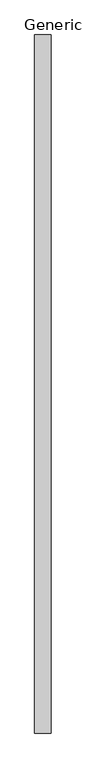
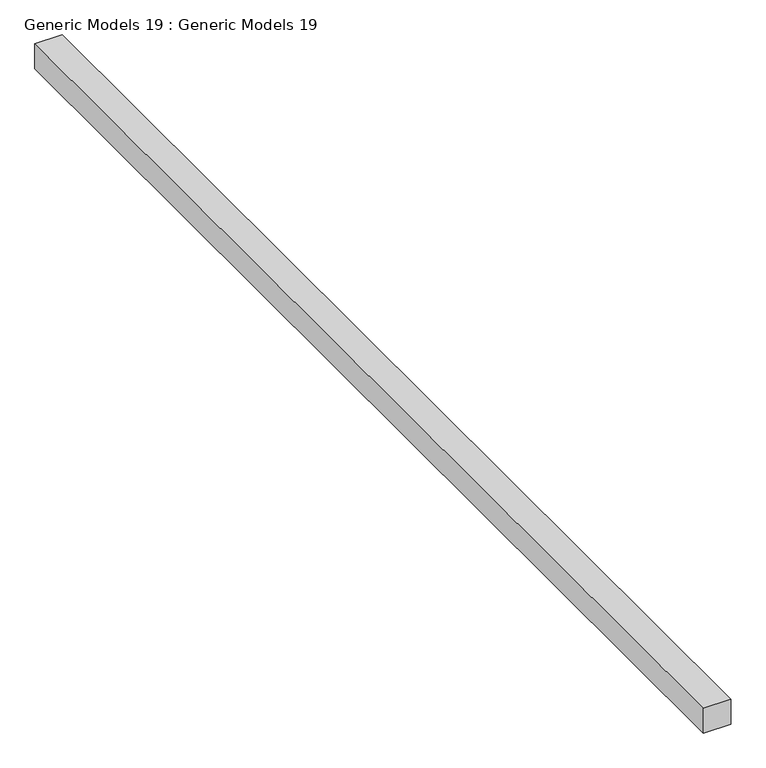
"""IFC4 building model written with IfcOpenShell, lengths in millimetres: proxy geometry, Generic Models 19 : Generic Models 19."""

from ifc_helpers import new_model, si_unit, frame, origin, place, context, project, spatial, polyline, outline, extrude, source, transform, mapped, element, save


def generic_models_19_generic_models_19_fbad5572(model_context):
    return source(origin(), model_context, "Body", "SweptSolid", [
        extrude(outline(polyline([(-15581.438074, -5966.8213044), (-15581.438074, 6932.2906387), (-15276.638074, 6932.2906387), (-15276.638074, -5966.8213044), (-15581.438074, -5966.8213044)])), frame((0.0, 0.0, 16154.4), z_axis=(0.0, 0.0, 1.0), x_axis=(1.0, 0.0, 0.0)), (0.0, 0.0, 1.0), 289.8499754),
    ])


if __name__ == "__main__":
    model = new_model("IFC4")
    model_context = context("Model", 3, world=origin())
    ifc_project = project(units=[si_unit("LENGTHUNIT", "METRE", prefix="MILLI")], contexts=[model_context])
    site = spatial("IfcSite", under=ifc_project)
    building = spatial("IfcBuilding", under=site)
    placement = place(None, origin())
    generic_models_19_generic_models_19_shape = generic_models_19_generic_models_19_fbad5572(model_context)
    element("IfcBuildingElementProxy", 1, Name="Generic Models 19 : Generic Models 19", ObjectType="Generic Models 19 : Generic Models 19", at=placement, inside=building, context=model_context, shape_type="MappedRepresentation", body=[
        mapped(generic_models_19_generic_models_19_shape, transform((0.0, 0.0, 0.0), x_axis=(1.0, 0.0, 0.0), y_axis=(0.0, 1.0, 0.0), z_axis=(0.0, 0.0, 1.0))),
    ])
    save(model, "model.ifc")
